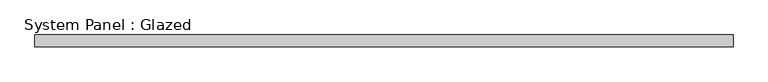
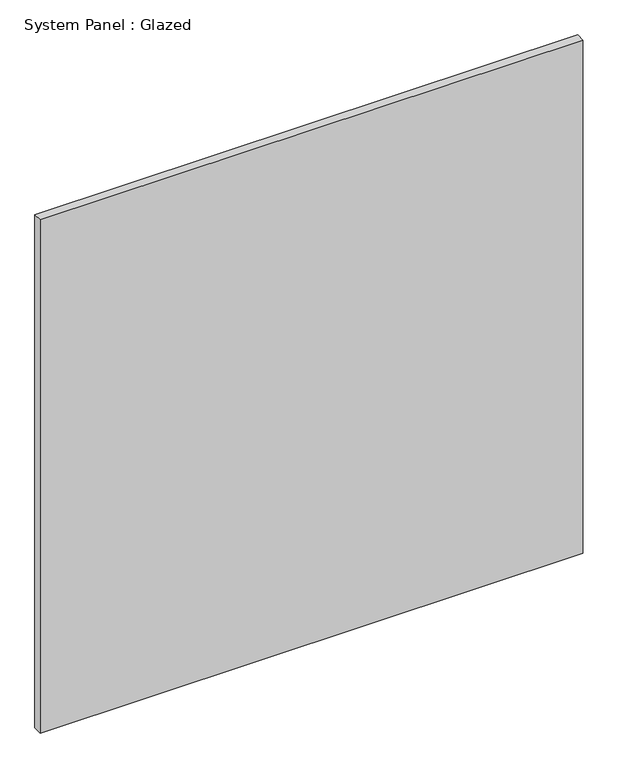
"""IFC4 building model written with IfcOpenShell, lengths in millimetres: plate geometry, System Panel : Glazed."""

from ifc_helpers import new_model, si_unit, origin, origin_with_axes, place, context, project, spatial, polyline, outline, extrude, source, transform, mapped, element, save


def system_panel_glazed_afe70ed6(model_context):
    return source(origin(), model_context, "Body", "SweptSolid", [
        extrude(outline(polyline([(762.0, 19.05), (-762.0, 19.05), (-762.0, 44.45), (762.0, 44.45), (762.0, 19.05)])), origin_with_axes(), (0.0, 0.0, 1.0), 1524.0),
    ])


if __name__ == "__main__":
    model = new_model("IFC4")
    model_context = context("Model", 3, world=origin())
    ifc_project = project(units=[si_unit("LENGTHUNIT", "METRE", prefix="MILLI")], contexts=[model_context])
    site = spatial("IfcSite", under=ifc_project)
    building = spatial("IfcBuilding", under=site)
    placement = place(None, origin())
    system_panel_glazed_shape = system_panel_glazed_afe70ed6(model_context)
    element("IfcPlate", 1, ObjectType="System Panel : Glazed", at=placement, inside=building, context=model_context, shape_type="MappedRepresentation", body=[
        mapped(system_panel_glazed_shape, transform((0.0, 0.0, 0.0), x_axis=(1.0, 0.0, 0.0), y_axis=(0.0, 1.0, 0.0), z_axis=(0.0, 0.0, 1.0))),
    ])
    save(model, "model.ifc")

# Revit data of these elements
# Type "System Panel : Glazed"
#   Construction Type Id = "GSP4R"
#   Analytic Construction = "1/8 in Pilkington single glazing"
#   Visual Light Transmittance = 0.9
#   Solar Heat Gain Coefficient = 0.86
#   Heat Transfer Coefficient (U) = 1.18115 BTU/(h·ft²·°F)
#   Define Thermal Properties by = 1
# Element 1 (IfcPlate, "System Panel : Glazed")
#   Materials on its faces: "Glass"
# Materials
#   "Glass": class "Glass", colour RGB 0 128 192, transparency 0.75, Description = "Soda Lime Glass", Cost = 0
